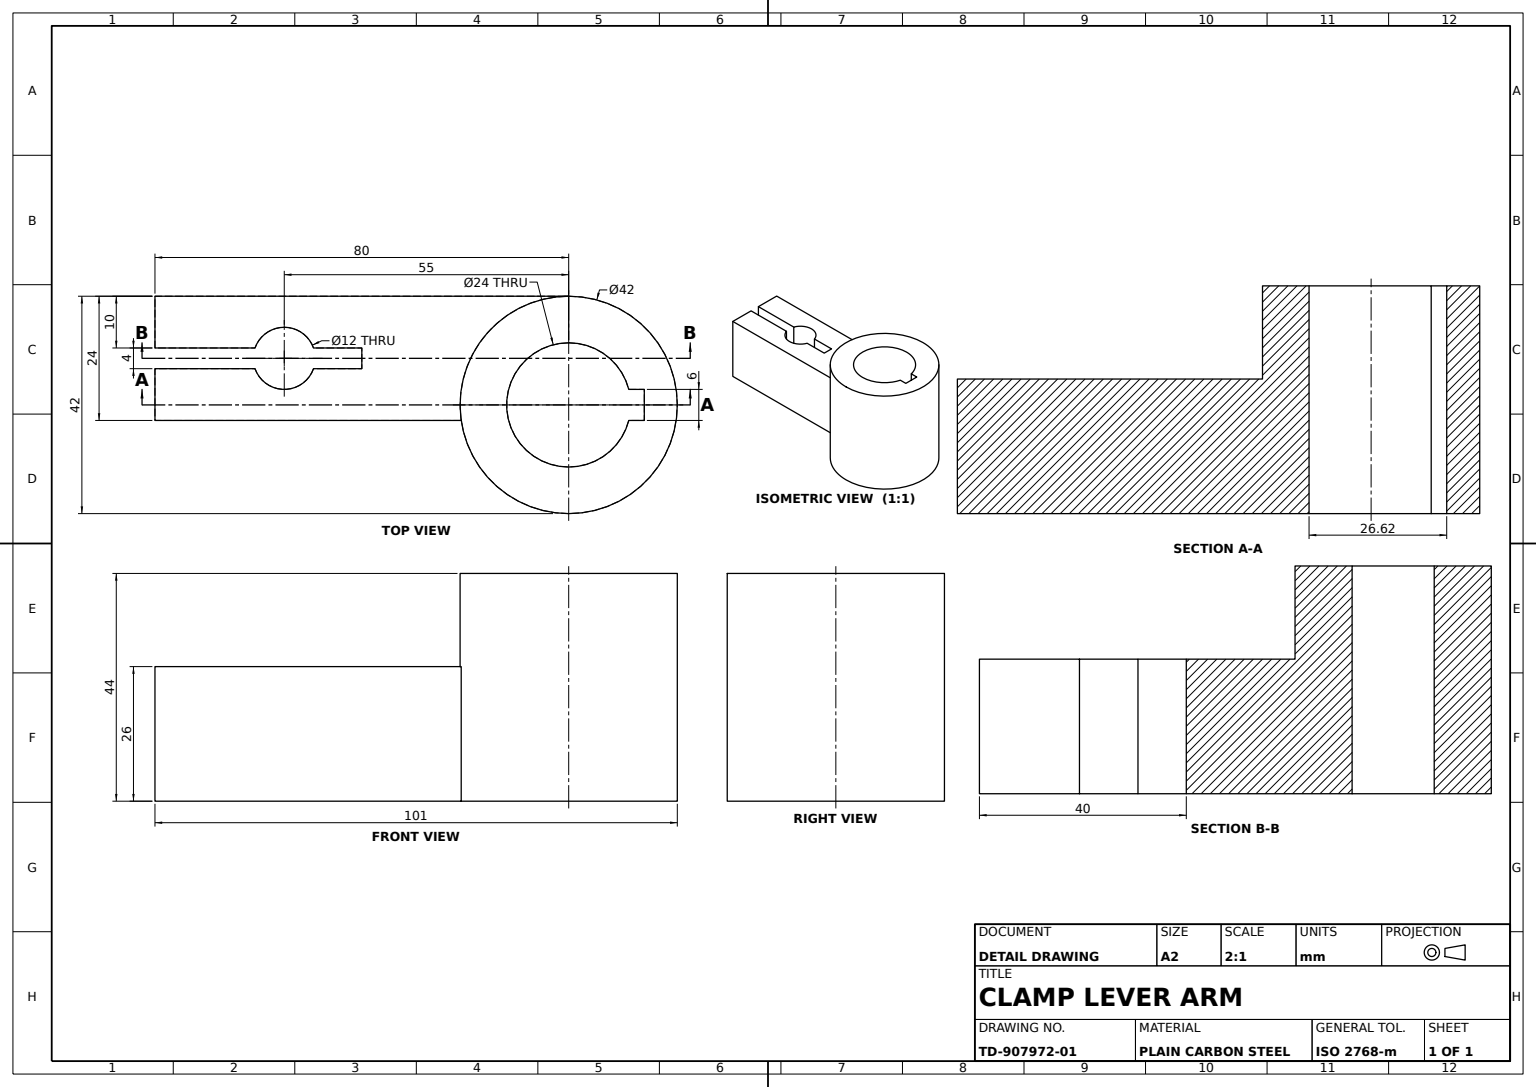
from build123d import *

# Parameters (mm, degrees)
LEVER_PROFILE_SKETCH_R      = 21
HUB_BOSS_44MM_DEPTH         = 44
SLOTTED_ARM_BOSS_26MM_DEPTH = 26


with BuildPart() as part:
    # Lever Profile Sketch → Hub Boss 44mm (new body)
    with BuildSketch(Plane(origin=(0, 0, 0), x_dir=(1, 0, 0), z_dir=(0, 1, 0))):
        with Locations(Location((0, 0, 0), (0, 0, 270))):
            Circle(LEVER_PROFILE_SKETCH_R)
        with BuildLine():
            Line((11.618950039, 3), (14.618950039, 3))
            Line((14.618950039, 3), (14.618950039, -3))
            Line((14.618950039, -3), (11.618950039, -3))
            ThreePointArc((11.618950039, -3), (-12, 0), (11.618950039, 3))
        make_face(mode=Mode.SUBTRACT)
    extrude(amount=HUB_BOSS_44MM_DEPTH)

    # Sketch1_3 → Slotted Arm Boss 26mm (add)
    with BuildSketch(Plane(origin=(0, 0, 0), x_dir=(1, 0, 0), z_dir=(0, 1, 0))):
        with BuildLine():
            ThreePointArc((-20.784609691, -3), (-15.874507866, 13.747727085), (0, 21))
            Line((0, 21), (-80, 21))
            Line((-80, 21), (-80, 11))
            Line((-80, 11), (-60.656854249, 11))
            ThreePointArc((-60.656854249, 11), (-55, 15), (-49.343145751, 11))
            Line((-49.343145751, 11), (-40, 11))
            Line((-40, 11), (-40, 7))
            Line((-40, 7), (-49.343145751, 7))
            ThreePointArc((-49.343145751, 7), (-55, 3), (-60.656854249, 7))
            Line((-60.656854249, 7), (-80, 7))
            Line((-80, 7), (-80, -3))
            Line((-80, -3), (-20.784609691, -3))
        make_face()
    extrude(amount=SLOTTED_ARM_BOSS_26MM_DEPTH)


solid = part.part
